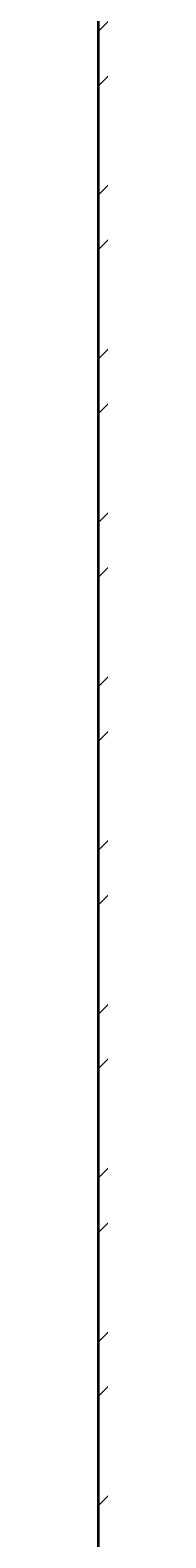
# Model space of a CAD drawing. Units: inches. Extents: x 1962 to 2771, y 1245 to 2660.
# Tile 89 of 114: x 2371 to 2371, y 2180 to 2304. Entities that reach past the tile are written whole.
import ezdxf

# ---------------------------------------------------------------- set-up
doc = ezdxf.new("R2010")
doc.units = ezdxf.units.IN
for name, color, linetype, lineweight in [('A-ANNO-DIMS', 2, 'Continuous', 18), ('A-WALL', 7, 'Continuous', 35), ('A-WALL-PATT', 252, 'Continuous', 13)]:
    doc.layers.add(name, color=color, linetype=linetype, lineweight=lineweight)
doc.styles.get("Standard").update_dxf_attribs({"font": 'arial.ttf'})
doc.dimstyles.get("Standard").update_dxf_attribs({"dimtxt": 0.18, "dimasz": 0.18, "dimexe": 0.18, "dimexo": 0.0625, "dimgap": 0.09, "dimtad": 0, "dimtih": 1, "dimtoh": 1, "dimdec": 4, "dimzin": 0, "dimdsep": 46, "dimtxsty": 'Standard', "dimcen": 0.09, "dimadec": 0, "dimazin": 0, "dimtfac": 1, "dimtdec": 4, "dimtofl": 0, "dimtmove": 0, "dimatfit": 3, "dimfxl": 1, "dimtolj": 1, "dimtzin": 0, "dimarcsym": 0})

# ---------------------------------------------------------------- blocks, each defined once
blk = doc.blocks.new('*D40')
at = {"layer": 'A-ANNO-DIMS', "color": 0, "lineweight": -2, "transparency": 16777216}
for p, q in [((2072.02, 2033.91), (2072.02, 2583.47)), ((2660.81, 2524.41), (2660.81, 2583.47)), ((2072.2, 2583.29), (2366.02, 2583.29)), ((2660.63, 2583.29), (2366.81, 2583.29))]:
    blk.add_line(p, q, dxfattribs=at)
at = {"layer": 'A-ANNO-DIMS', "color": 0, "transparency": 16777216}
for points in [[(2072.2, 2583.32), (2072.2, 2583.26), (2072.02, 2583.29)], [(2660.63, 2583.32), (2660.63, 2583.26), (2660.81, 2583.29)]]:
    blk.add_solid(points, dxfattribs=at)
at = {"layer": 'Defpoints', "color": 0, "transparency": 16777216}
for p in [(2660.81, 2583.29), (2660.81, 2524.34), (2072.02, 2033.84)]:
    blk.add_point(p, dxfattribs=at)
at = {"layer": 'A-ANNO-DIMS', "color": 0, "transparency": 16777216, "insert": (2366.41, 2583.29), "char_height": 0.18, "attachment_point": 5}
blk.add_mtext('\\A1;588.8', dxfattribs=at)

msp = doc.modelspace()

# ---------------------------------------------------------------- hatches: boundary and pattern name
at = {"layer": 'A-WALL-PATT'}
h = msp.add_hatch(dxfattribs=at)
h.set_pattern_fill('ANSI32', color=256)
h.paths.add_polyline_path([(2090.8074, 2467.3437), (2141.6481, 2467.3437), (2141.6481, 2469.5937), (2141.6481, 2471.8437), (2086.3074, 2471.8437), (2086.3074, 2422.5333), (2090.8074, 2422.5333)])
h.paths.add_polyline_path([(2282.7664, 2471.8437), (2204.8982, 2471.8437), (2204.8982, 2467.3437), (2234.8074, 2467.3437), (2234.8074, 2311.3437), (2228.7492, 2311.3437), (2228.7492, 2306.8437), (2234.8074, 2306.8437), (2331.9227, 2306.8437), (2331.9227, 2309.0937), (2331.9227, 2311.3437), (2239.3074, 2311.3437), (2239.3074, 2467.3437), (2282.7664, 2467.3437), (2282.7664, 2469.5937)])
h.paths.add_polyline_path([(2471.4531, 2519.8437), (2552.011, 2519.8437), (2564.3996, 2519.8437), (2564.3996, 2511.1389), (2568.8996, 2511.1389), (2568.8996, 2524.3437), (2466.9531, 2524.3437), (2466.9531, 2471.8437), (2450.0749, 2471.8437), (2446.4672, 2471.8437), (2446.4672, 2467.3437), (2450.0749, 2467.3437), (2475.9988, 2467.3437), (2475.9988, 2469.5937), (2475.9988, 2471.8437), (2471.4531, 2471.8437)])
h.paths.add_polyline_path([(2575.2231, 2469.5937), (2575.2231, 2471.8437), (2568.8996, 2471.8437), (2568.8996, 2487.1389), (2564.3996, 2487.1389), (2564.3996, 2471.8437), (2556.511, 2471.8437), (2499.2904, 2471.8437), (2499.2904, 2467.3437), (2507.8074, 2467.3437), (2507.8074, 2311.3437), (2414.863, 2311.3437), (2414.863, 2306.8437), (2512.3074, 2306.8437), (2517.0114, 2306.8437), (2517.0114, 2309.0937), (2517.0114, 2311.3437), (2512.3074, 2311.3437), (2512.3074, 2467.3437), (2575.2231, 2467.3437)])
h.paths.add_polyline_path([(2660.8074, 2471.8437), (2600.9602, 2471.8437), (2600.9602, 2467.3437), (2656.3074, 2467.3437), (2656.3074, 2432.5704), (2660.8074, 2432.5704)])
h.paths.add_polyline_path([(2660.8074, 2372.5704), (2656.3074, 2372.5704), (2656.3074, 2311.3437), (2600.276, 2311.3437), (2600.276, 2309.0937), (2600.276, 2306.8437), (2656.3074, 2306.8437), (2656.3074, 2296.2593), (2660.8074, 2296.2593)])
h.paths.add_polyline_path([(2572.3074, 2306.8437), (2577.1385, 2306.8437), (2577.1385, 2311.3437), (2551.082, 2311.3437), (2551.082, 2306.8437), (2567.8074, 2306.8437), (2567.8074, 2258.8437), (2540.0574, 2258.8437), (2540.0574, 2256.5937), (2540.0574, 2254.3437), (2567.8074, 2254.3437), (2656.3074, 2254.3437), (2656.3074, 2236.9085), (2660.8074, 2236.9085), (2660.8074, 2272.2593), (2656.3074, 2272.2593), (2656.3074, 2258.8437), (2572.3074, 2258.8437)])
h.paths.add_polyline_path([(2512.3074, 2254.3437), (2518.8716, 2254.3437), (2518.8716, 2256.5937), (2518.8716, 2258.8437), (2507.8074, 2258.8437), (2507.8074, 2177.8437), (2567.8074, 2177.8437), (2567.8074, 2172.9628), (2572.3074, 2172.9628), (2572.3074, 2177.8437), (2656.3074, 2177.8437), (2656.3074, 2166.4846), (2660.8074, 2166.4846), (2660.8074, 2200.9085), (2656.3074, 2200.9085), (2656.3074, 2182.3437), (2512.3074, 2182.3437)])
h.paths.add_polyline_path([(2656.3074, 2129.8437), (2572.3074, 2129.8437), (2572.3074, 2150.3044), (2570.0574, 2150.3044), (2567.8074, 2150.3044), (2567.8074, 2129.8437), (2507.8074, 2129.8437), (2507.8074, 2116.3027), (2510.0574, 2116.3027), (2512.3074, 2116.3027), (2512.3074, 2125.3437), (2567.8074, 2125.3437), (2572.3074, 2125.3437), (2656.3074, 2125.3437)])
h.paths.add_polyline_path([(2090.8074, 2362.5333), (2086.3074, 2362.5333), (2086.3074, 2298.6242), (2090.8074, 2298.6242), (2090.8074, 2306.8437), (2174.8074, 2306.8437), (2174.8074, 2286.4178), (2179.3074, 2286.4178), (2179.3074, 2306.8437), (2192.8641, 2306.8437), (2192.8641, 2309.0937), (2192.8641, 2311.3437), (2090.8074, 2311.3437)])
h.paths.add_polyline_path([(2209.156, 2258.8437), (2179.3074, 2258.8437), (2179.3074, 2263.2236), (2177.0574, 2263.2236), (2174.8074, 2263.2236), (2174.8074, 2258.8437), (2090.8074, 2258.8437), (2090.8074, 2274.6242), (2086.3074, 2274.6242), (2086.3074, 2238.2967), (2088.5574, 2238.2967), (2090.8074, 2238.2967), (2090.8074, 2254.3437), (2209.156, 2254.3437)])
h.paths.add_polyline_path([(2090.8074, 2177.8437), (2234.8074, 2177.8437), (2234.8074, 2173.1428), (2239.3074, 2173.1428), (2239.3074, 2258.8437), (2230.8442, 2258.8437), (2230.8442, 2256.5937), (2230.8442, 2254.3437), (2234.8074, 2254.3437), (2234.8074, 2182.3437), (2090.8074, 2182.3437), (2090.8074, 2202.2967), (2086.3074, 2202.2967), (2086.3074, 2140.0389), (2090.8074, 2140.0389)])
h.paths.add_polyline_path([(2090.8074, 2080.0389), (2086.3074, 2080.0389), (2086.3074, 2033.8437), (2090.8074, 2033.8437)], flags=17)
h.paths.add_polyline_path([(2244.9405, 2033.8437), (2239.3074, 2033.8437), (2239.3074, 2142.0665), (2237.2592, 2142.0665), (2234.8074, 2142.0665), (2234.8074, 2033.8437), (2090.8074, 2033.8437), (2076.5204, 2033.8437), (2072.0204, 2033.8437), (2072.0204, 2000.4493), (2076.5204, 2000.4493), (2076.5204, 2029.3437), (2090.8074, 2029.3437), (2244.9405, 2029.3437), (2244.9405, 2031.5937)])
h.paths.add_polyline_path([(2234.8074, 1933.3437), (2076.5204, 1933.3437), (2076.5204, 1952.4493), (2074.2704, 1952.4493), (2072.0204, 1952.4493), (2072.0204, 1933.3437), (2072.0204, 1928.8437), (2234.8074, 1928.8437)])
h.paths.add_polyline_path([(2090.8074, 1928.8437), (2086.3074, 1928.8437), (2086.3074, 1906.5013), (2090.8074, 1906.5013)])
h.paths.add_polyline_path([(2090.8074, 1846.5013), (2086.3074, 1846.5013), (2086.3074, 1769.9917), (2088.5574, 1769.9917), (2090.8074, 1769.9917), (2090.8074, 1780.3437), (2234.8074, 1780.3437), (2234.8074, 1708.3437), (2230.3764, 1708.3437), (2230.3764, 1703.8437), (2239.3074, 1703.8437), (2239.3074, 1792.6669), (2237.0574, 1792.6669), (2234.8074, 1792.6669), (2234.8074, 1784.8437), (2090.8074, 1784.8437)])
h.paths.add_polyline_path([(2239.3074, 1928.8437), (2244.9405, 1928.8437), (2244.9405, 1931.0937), (2244.9405, 1933.3437), (2234.8074, 1933.3437), (2234.8074, 1928.8437), (2234.8074, 1825.5949), (2239.3074, 1825.5949)])
h.paths.add_polyline_path([(2148.0425, 1649.0937), (2148.0425, 1651.3437), (2090.8074, 1651.3437), (2090.8074, 1646.8437), (2148.0425, 1646.8437)], flags=0)
h.paths.add_polyline_path([(2207.5601, 1708.3437), (2090.8074, 1708.3437), (2090.8074, 1703.8437), (2174.8074, 1703.8437), (2174.8074, 1651.3437), (2170.4457, 1651.3437), (2170.4457, 1646.8437), (2195.9924, 1646.8437), (2195.9924, 1649.0937), (2195.9924, 1651.3437), (2179.3074, 1651.3437), (2179.3074, 1703.8437), (2207.5601, 1703.8437), (2207.5601, 1706.0937)])
h.paths.add_polyline_path([(2090.8074, 1733.9917), (2086.3074, 1733.9917), (2086.3074, 1696.1032), (2088.5574, 1696.1032), (2090.8074, 1696.1032)])
h.paths.add_polyline_path([(2090.8074, 1672.1032), (2086.3074, 1672.1032), (2086.3074, 1600.3335), (2090.8074, 1600.3335)])
h.paths.add_polyline_path([(2090.8074, 1540.3335), (2086.3074, 1540.3335), (2086.3074, 1486.3437), (2139.6766, 1486.3437), (2139.6766, 1490.8437), (2090.8074, 1490.8437)])
h.paths.add_polyline_path([(2302.3876, 1490.8437), (2239.3074, 1490.8437), (2239.3074, 1646.8437), (2335.9994, 1646.8437), (2335.9994, 1651.3437), (2229.884, 1651.3437), (2229.884, 1646.8437), (2234.8074, 1646.8437), (2234.8074, 1490.8437), (2202.7103, 1490.8437), (2202.7103, 1488.5937), (2202.7103, 1486.3437), (2275.0699, 1486.3437), (2275.0699, 1475.772), (2279.5699, 1475.772), (2279.5699, 1486.3437), (2302.3876, 1486.3437)])
h.paths.add_polyline_path([(2279.5699, 1451.772), (2275.0699, 1451.772), (2275.0699, 1438.3437), (2174.8074, 1438.3437), (2174.8074, 1486.3437), (2179.7922, 1486.3437), (2179.7922, 1490.8437), (2163.3585, 1490.8437), (2163.3585, 1488.5937), (2163.3585, 1486.3437), (2170.3074, 1486.3437), (2170.3074, 1433.8437), (2279.5699, 1433.8437)])
h.paths.add_polyline_path([(2427.2363, 1490.8437), (2375.8074, 1490.8437), (2375.8074, 1646.8437), (2381.6401, 1646.8437), (2381.6401, 1651.3437), (2365.887, 1651.3437), (2365.887, 1649.0937), (2365.887, 1646.8437), (2371.3074, 1646.8437), (2371.3074, 1490.8437), (2327.5627, 1490.8437), (2327.5627, 1488.5937), (2327.5627, 1486.3437), (2371.3074, 1486.3437), (2371.3074, 1433.8437), (2375.8074, 1433.8437), (2375.8074, 1486.3437), (2427.2363, 1486.3437)])
h.paths.add_polyline_path([(2512.3074, 1646.8437), (2519.4351, 1646.8437), (2519.4351, 1649.0937), (2519.4351, 1651.3437), (2507.8074, 1651.3437), (2416.0063, 1651.3437), (2416.0063, 1649.0937), (2416.0063, 1646.8437), (2507.8074, 1646.8437), (2507.8074, 1490.8437), (2497.0532, 1490.8437), (2497.0532, 1488.5937), (2497.0532, 1486.3437), (2574.9344, 1486.3437), (2574.9344, 1476.0181), (2579.4344, 1476.0181), (2579.4344, 1486.3437), (2584.4872, 1486.3437), (2584.3074, 1490.8437), (2512.3074, 1490.8437)])
h.paths.add_polyline_path([(2470.5091, 1486.3437), (2473.9767, 1486.3437), (2473.9767, 1490.8437), (2449.6605, 1490.8437), (2449.6605, 1488.5937), (2449.6605, 1486.3437), (2466.0091, 1486.3437), (2466.0091, 1433.8437), (2470.5091, 1433.8437), (2579.4344, 1433.8437), (2579.4344, 1452.0181), (2574.9344, 1452.0181), (2574.9344, 1438.3437), (2554.5091, 1438.3437), (2470.5091, 1438.3437)])
h.paths.add_polyline_path([(2656.3074, 1490.8437), (2611.86, 1490.8437), (2611.86, 1486.3437), (2656.3074, 1486.3437)])
h.paths.add_polyline_path([(2660.8074, 1532.7007), (2658.5574, 1532.7007), (2656.3074, 1532.7007), (2656.3074, 1486.3437), (2660.8074, 1486.3437)])
h.paths.add_polyline_path([(2660.8074, 1664.9663), (2656.3074, 1664.9663), (2656.3074, 1651.3437), (2602.2313, 1651.3437), (2602.2313, 1646.8437), (2656.3074, 1646.8437), (2656.3074, 1592.7007), (2660.8074, 1592.7007)])
h.paths.add_polyline_path([(2660.8074, 1724.5221), (2656.3074, 1724.5221), (2656.3074, 1703.8437), (2542.4725, 1703.8437), (2542.4725, 1699.3437), (2567.8074, 1699.3437), (2567.8074, 1651.3437), (2552.7766, 1651.3437), (2552.7766, 1649.0937), (2552.7766, 1646.8437), (2577.2878, 1646.8437), (2577.2878, 1649.0937), (2577.2878, 1651.3437), (2572.3074, 1651.3437), (2572.3074, 1699.3437), (2656.3074, 1699.3437), (2656.3074, 1688.9663), (2660.8074, 1688.9663)])
h.paths.add_polyline_path([(2660.8074, 1880.6524), (2656.3074, 1880.6524), (2656.3074, 1832.8437), (2512.3074, 1832.8437), (2512.3074, 1837.8959), (2507.8074, 1837.8959), (2507.8074, 1828.3437), (2567.8074, 1828.3437), (2567.8074, 1804.3437), (2572.3074, 1804.3437), (2572.3074, 1828.3437), (2656.3074, 1828.3437), (2656.3074, 1818.6778), (2660.8074, 1818.6778)])
h.paths.add_polyline_path([(2660.8074, 1794.6778), (2656.3074, 1794.6778), (2656.3074, 1780.3437), (2572.3074, 1780.3437), (2572.3074, 1783.0303), (2570.0574, 1783.0303), (2567.8074, 1783.0303), (2567.8074, 1780.3437), (2507.8074, 1780.3437), (2507.8074, 1699.3437), (2517.8858, 1699.3437), (2517.8858, 1701.5937), (2517.8858, 1703.8437), (2512.3074, 1703.8437), (2512.3074, 1775.8437), (2656.3074, 1775.8437), (2656.3074, 1760.5221), (2660.8074, 1760.5221)])
h.paths.add_polyline_path([(2660.8074, 1981.3437), (2660.8074, 2020.2808), (2658.5574, 2020.2808), (2656.3074, 2020.2808), (2656.3074, 1981.3437), (2512.3074, 1981.3437), (2512.3074, 2086.6996), (2507.8074, 2086.6996), (2507.8074, 1981.3437), (2375.8074, 1981.3437), (2375.8074, 1986.8505), (2373.5574, 1986.8505), (2371.3074, 1986.8505), (2371.3074, 1973.2607), (2375.8074, 1973.2607), (2375.8074, 1976.8437), (2507.8074, 1976.8437), (2507.8074, 1865.4281), (2510.0574, 1865.4281), (2512.3074, 1865.4281), (2512.3074, 1976.8437), (2660.8074, 1976.8437)])
h.paths.add_polyline_path([(2375.8074, 1940.297), (2373.5574, 1940.297), (2371.3074, 1940.297), (2371.3074, 1933.3437), (2278.4434, 1933.3437), (2278.4434, 1928.8437), (2371.3074, 1928.8437), (2371.3074, 1651.3437), (2375.8074, 1651.3437)])
h.paths.add_polyline_path([(2660.8074, 1976.8437), (2656.3074, 1976.8437), (2656.3074, 1940.6524), (2660.8074, 1940.6524)], flags=17)
h.paths.add_polyline_path([(2660.8074, 2142.4846), (2656.3074, 2142.4846), (2656.3074, 2080.2808), (2660.8074, 2080.2808)])
h.paths.add_polyline_path([(2381.4189, 2311.3437), (2375.8074, 2311.3437), (2375.8074, 2467.3437), (2424.7242, 2467.3437), (2424.7242, 2469.5937), (2424.7242, 2471.8437), (2375.8074, 2471.8437), (2375.8074, 2524.3437), (2371.3074, 2524.3437), (2371.3074, 2471.8437), (2307.2097, 2471.8437), (2307.2097, 2467.3437), (2371.3074, 2467.3437), (2371.3074, 2311.3437), (2366.8901, 2311.3437), (2366.8901, 2306.8437), (2371.3074, 2306.8437), (2371.3074, 2033.8437), (2279.6589, 2033.8437), (2279.6589, 2029.3437), (2371.3074, 2029.3437), (2371.3074, 2014.2598), (2375.8074, 2014.2598), (2375.8074, 2306.8437), (2381.4189, 2306.8437)])
h.paths.add_polyline_path([(2263.3074, 2524.3437), (2170.3074, 2524.3437), (2170.3074, 2519.8437), (2170.3074, 2471.8437), (2165.0312, 2471.8437), (2165.0312, 2467.3437), (2179.6721, 2467.3437), (2179.6721, 2469.5161), (2179.6721, 2471.8437), (2174.8074, 2471.8437), (2174.8074, 2519.8437), (2258.8074, 2519.8437), (2258.8074, 2511.6436), (2263.3074, 2511.6436)])
h.paths.add_polyline_path([(2245.0232, 1361.4123), (2492.9468, 1361.4123), (2492.9468, 1398.505), (2245.0232, 1398.505)], flags=9)
h.paths.add_polyline_path([(2388.1434, 2086.6936), (2425.0704, 2086.6936), (2425.0704, 2105.3509), (2388.1434, 2105.3509)], flags=9)
h.paths.add_polyline_path([(2404.922, 2242.6744), (2445.7337, 2242.6744), (2445.7337, 2261.3318), (2404.922, 2261.3318)], flags=9)
h.paths.add_polyline_path([(2269.4107, 2156.7935), (2306.3378, 2156.7935), (2306.3378, 2175.4508), (2269.4107, 2175.4508)], flags=9)
h.paths.add_polyline_path([(2269.3277, 2233.4343), (2306.2547, 2233.4343), (2306.2547, 2252.0917), (2269.3277, 2252.0917)], flags=9)
h.paths.add_polyline_path([(2431.6052, 2320.6922), (2470.4456, 2320.6922), (2470.4456, 2339.3495), (2431.6052, 2339.3495)], flags=25)
h.paths.add_polyline_path([(2249.6902, 2315.7608), (2288.5306, 2315.7608), (2288.5306, 2334.4182), (2249.6902, 2334.4182)], flags=25)
h.paths.add_polyline_path([(2096.9301, 2314.3181), (2135.7704, 2314.3181), (2135.7704, 2332.9755), (2096.9301, 2332.9755)], flags=25)
h.paths.add_polyline_path([(2134.3475, 2285.7089), (2161.4655, 2285.7089), (2161.4655, 2304.3662), (2134.3475, 2304.3662)], flags=9)
h.paths.add_polyline_path([(2126.5155, 2209.4076), (2159.9227, 2209.4076), (2159.9227, 2228.065), (2126.5155, 2228.065)], flags=25)
h.paths.add_polyline_path([(2110.5753, 2141.5299), (2149.4157, 2141.5299), (2149.4157, 2160.1872), (2110.5753, 2160.1872)], flags=25)
h.paths.add_polyline_path([(2249.8618, 1968.3317), (2286.3966, 1968.3317), (2286.3966, 1986.989), (2249.8618, 1986.989)], flags=9)
h.paths.add_polyline_path([(2395.9507, 1777.0051), (2436.7624, 1777.0051), (2436.7624, 1795.6625), (2395.9507, 1795.6625)], flags=9)
h.paths.add_polyline_path([(2398.5259, 1888.5651), (2435.0062, 1888.5651), (2435.0062, 1907.2224), (2398.5259, 1907.2224)], flags=25)
h.paths.add_polyline_path([(2259.3506, 1728.3559), (2296.2776, 1728.3559), (2296.2776, 1747.0132), (2259.3506, 1747.0132)], flags=9)
h.paths.add_polyline_path([(2271.3698, 1845.268), (2308.2968, 1845.268), (2308.2968, 1863.9253), (2271.3698, 1863.9253)], flags=9)
h.paths.add_polyline_path([(2120.9355, 1786.3027), (2159.7759, 1786.3027), (2159.7759, 1804.9601), (2120.9355, 1804.9601)], flags=25)
h.paths.add_polyline_path([(2121.3164, 1732.1043), (2154.7236, 1732.1043), (2154.7236, 1750.7616), (2121.3164, 1750.7616)], flags=25)
h.paths.add_polyline_path([(2118.3706, 1678.8997), (2147.5282, 1678.8997), (2147.5282, 1697.557), (2118.3706, 1697.557)], flags=25)
h.paths.add_polyline_path([(2385.9227, 1493.557), (2424.763, 1493.557), (2424.763, 1512.2143), (2385.9227, 1512.2143)], flags=25)
h.paths.add_polyline_path([(2248.7058, 1500.0256), (2287.5462, 1500.0256), (2287.5462, 1518.6829), (2248.7058, 1518.6829)], flags=25)
h.paths.add_polyline_path([(2104.1669, 1617.3771), (2143.0073, 1617.3771), (2143.0073, 1636.0344), (2104.1669, 1636.0344)], flags=9)
h.paths.add_polyline_path([(2096.0714, 1447.8824), (2137.3845, 1447.8824), (2137.3845, 1458.1859), (2096.0714, 1458.1859)], flags=9)
h.paths.add_polyline_path([(2180.6114, 1440.325), (2209.7689, 1440.325), (2209.7689, 1458.9823), (2180.6114, 1458.9823)], flags=25)
h.paths.add_polyline_path([(2316.1698, 1447.9637), (2357.4829, 1447.9637), (2357.4829, 1458.2673), (2316.1698, 1458.2673)], flags=9)
h.paths.add_polyline_path([(2397.6187, 1447.9637), (2438.9318, 1447.9637), (2438.9318, 1458.2673), (2397.6187, 1458.2673)], flags=9)
h.paths.add_polyline_path([(2473.0778, 1439.5953), (2502.2354, 1439.5953), (2502.2354, 1458.2527), (2473.0778, 1458.2527)], flags=25)
h.paths.add_polyline_path([(2589.7027, 1447.8819), (2631.0158, 1447.8819), (2631.0158, 1458.1855), (2589.7027, 1458.1855)], flags=9)
h.paths.add_polyline_path([(2522.4009, 1497.5285), (2561.2413, 1497.5285), (2561.2413, 1516.1859), (2522.4009, 1516.1859)], flags=25)
h.paths.add_polyline_path([(2579.6565, 1671.3482), (2608.8141, 1671.3482), (2608.8141, 1690.0056), (2579.6565, 1690.0056)], flags=25)
h.paths.add_polyline_path([(2544.7038, 1725.5064), (2578.1111, 1725.5064), (2578.1111, 1744.1637), (2544.7038, 1744.1637)], flags=25)
h.paths.add_polyline_path([(2578.1191, 1807.472), (2607.2766, 1807.472), (2607.2766, 1826.1293), (2578.1191, 1826.1293)], flags=25)
h.paths.add_polyline_path([(2595.0614, 1835.1839), (2633.9018, 1835.1839), (2633.9018, 1853.8413), (2595.0614, 1853.8413)], flags=25)
h.paths.add_polyline_path([(2567.0097, 2097.7035), (2605.8501, 2097.7035), (2605.8501, 2116.3609), (2567.0097, 2116.3609)], flags=9)
h.paths.add_polyline_path([(2586.644, 2134.6454), (2615.8015, 2134.6454), (2615.8015, 2153.3027), (2586.644, 2153.3027)], flags=9)
h.paths.add_polyline_path([(2544.6185, 2212.6783), (2578.0258, 2212.6783), (2578.0258, 2231.3356), (2544.6185, 2231.3356)], flags=25)
h.paths.add_polyline_path([(2577.0273, 2256.9023), (2606.1849, 2256.9023), (2606.1849, 2275.5597), (2577.0273, 2275.5597)], flags=24)
h.paths.add_polyline_path([(2605.2683, 2315.2821), (2644.1087, 2315.2821), (2644.1087, 2333.9395), (2605.2683, 2333.9395)], flags=25)
h.paths.add_polyline_path([(2583.1244, 2496.1815), (2624.4375, 2496.1815), (2624.4375, 2506.4851), (2583.1244, 2506.4851)], flags=9)
h.paths.add_polyline_path([(2474.761, 2497.0823), (2503.9185, 2497.0823), (2503.9185, 2515.7397), (2474.761, 2515.7397)], flags=25)
h.paths.add_polyline_path([(2387.5787, 2494.2563), (2428.902, 2494.2563), (2428.902, 2504.5598), (2387.5787, 2504.5598)], flags=9)
h.paths.add_polyline_path([(2300.1657, 2500.1564), (2341.4788, 2500.1564), (2341.4788, 2510.46), (2300.1657, 2510.46)], flags=25)
h.paths.add_polyline_path([(2176.8589, 2497.5843), (2206.0165, 2497.5843), (2206.0165, 2516.2416), (2176.8589, 2516.2416)], flags=25)
h.paths.add_polyline_path([(2097.4668, 2494.9762), (2138.7799, 2494.9762), (2138.7799, 2505.2798), (2097.4668, 2505.2798)], flags=9)

# ---------------------------------------------------------------- linework, layer by layer
at = {"layer": 'A-WALL'}
msp.add_line((2371.3074, 2306.8437), (2371.3074, 2033.8437), dxfattribs=at)

# ---------------------------------------------------------------- dimensions: what is measured, and where the dimension line sits
at = {"layer": 'A-ANNO-DIMS'}
dim = msp.add_linear_dim(base=(2660.8074, 2583.2937), p1=(2072.0204, 2033.8437), p2=(2660.8074, 2524.3437), dimstyle='Standard', override={"dimdec": 1, "dimlfac": 1, "dimrnd": 0, "dimzin": 0, "dimdsep": 46, "dimlunit": 2}, dxfattribs=at)
dim.commit()
dim.dimension.update_dxf_attribs({"geometry": '*D40', "text_midpoint": (2366.4139, 2583.2937)})

doc.saveas('drawing.dxf')
